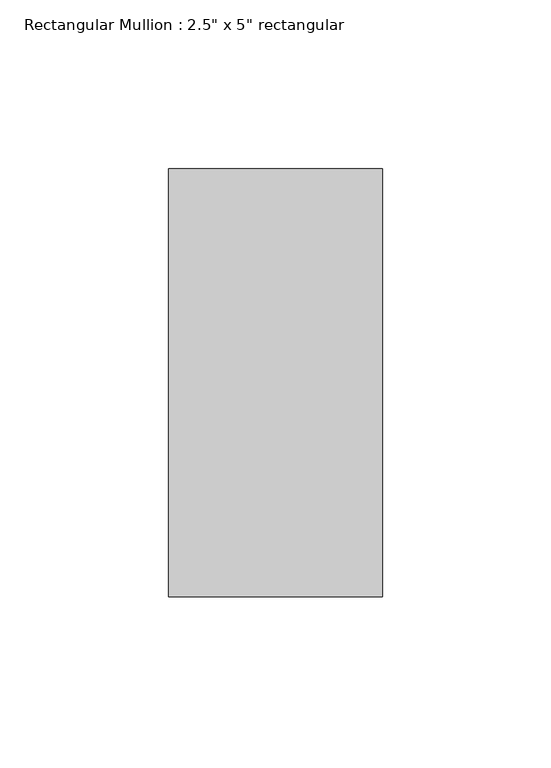
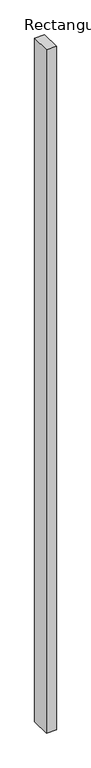
"""IFC4 building model written with IfcOpenShell, lengths in millimetres: member geometry."""

from ifc_helpers import new_model, si_unit, frame, origin, place, context, project, spatial, polyline, outline, extrude, source, transform, mapped, element, save


def member_f500ba6f(model_context):
    return source(origin(), model_context, "Body", "SweptSolid", [
        extrude(outline(polyline([(0.0, 63.5), (0.0, -63.5), (-63.5, -63.5), (-63.5, 63.5), (0.0, 63.5)])), frame((0.0, 0.0, -4567.1863081), z_axis=(0.0, 0.0, 1.0), x_axis=(1.0, 0.0, 0.0)), (0.0, 0.0, 1.0), 4567.1863081),
    ])


if __name__ == "__main__":
    model = new_model("IFC4")
    model_context = context("Model", 3, world=origin())
    ifc_project = project(units=[si_unit("LENGTHUNIT", "METRE", prefix="MILLI")], contexts=[model_context])
    site = spatial("IfcSite", under=ifc_project)
    building = spatial("IfcBuilding", under=site)
    placement = place(None, origin())
    member_shape = member_f500ba6f(model_context)
    element("IfcMember", 1, ObjectType="Rectangular Mullion : 2.5\" x 5\" rectangular", at=placement, inside=building, context=model_context, shape_type="MappedRepresentation", body=[
        mapped(member_shape, transform((0.0, 0.0, 0.0), x_axis=(1.0, 0.0, 0.0), y_axis=(0.0, 1.0, 0.0), z_axis=(0.0, 0.0, 1.0))),
    ])
    save(model, "model.ifc")

# Revit data of these elements
# Type "Rectangular Mullion : 2.5\" x 5\" rectangular"
#   built-in parameter 1007304 = 0.416667 (stored number, unit not read)
#   built-in parameter 1007301 = 0.104167 (stored number, unit not read)
#   built-in parameter 1007300 = 0.104167 (stored number, unit not read)
# Element 1 (IfcMember, "Rectangular Mullion : 2.5\" x 5\" rectangular")
#   Materials on its faces: "Aluminum"
# Materials
#   "Aluminum": class "Metal", colour RGB 247 247 247, transparency 0, Description = "Aluminum 6061", Cost = 0
